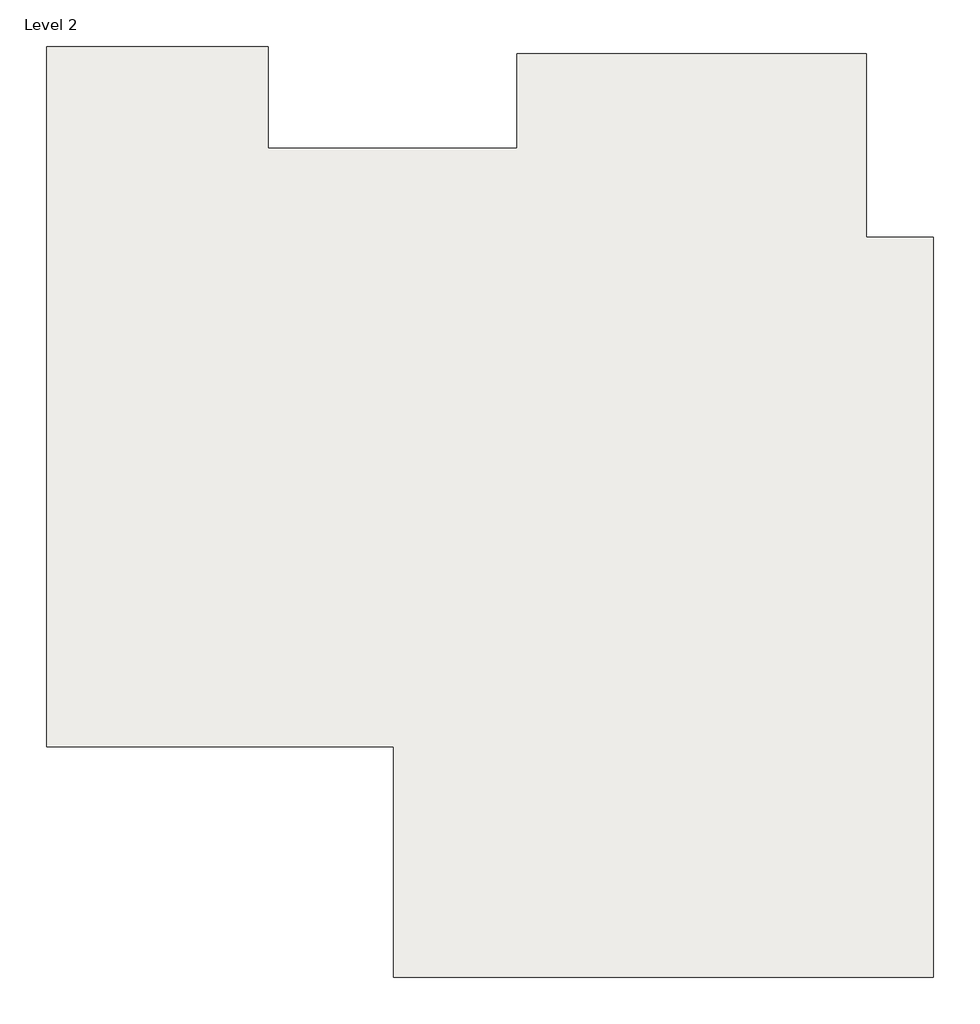
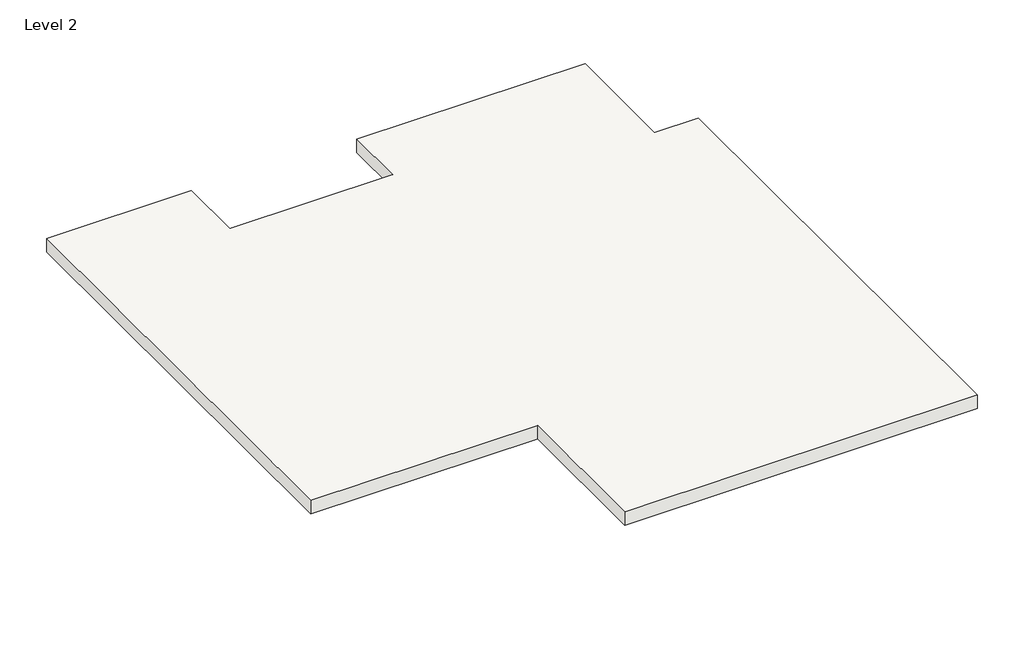
# One storey: 1 roof.
"""IFC4 building model written with IfcOpenShell, lengths in millimetres."""

from ifc_helpers import new_model, si_unit, frame, origin, place, context, project, spatial, polyline, outline, extrude, element, save

model = new_model("IFC4")

# Units and contexts
model_context = context("Model", 3, world=origin())
ifc_project = project(units=[si_unit("LENGTHUNIT", "METRE", prefix="MILLI")], contexts=[model_context])

# Site, building, storey
site = spatial("IfcSite", under=ifc_project)
building = spatial("IfcBuilding", under=site)
storey = spatial("IfcBuildingStorey", under=building, Name="Level 2", Elevation=3048.0)

# Roof
placement = place(None, origin())
element("IfcRoof", 1, ObjectType="Generic - 12\"", at=placement, inside=storey, context=model_context, shape_type="SweptSolid", body=[
    extrude(outline(polyline([(-12724.8234692, 10555.2116886), (-9626.0234692, 10555.2116886), (-9626.0234692, 9132.8116886), (-6146.2234692, 9132.8116886), (-6146.2234692, 10453.6116886), (-1269.4234692, 10453.6116886), (-1269.4234692, 7888.2116886), (-329.6234692, 7888.2116886), (-329.6234692, -2449.5883114), (-7873.4234692, -2449.5883114), (-7873.4234692, 776.2116886), (-12724.8234692, 776.2116886), (-12724.8234692, 10555.2116886)])), frame((0.0, 0.0, 3048.0), z_axis=(0.0, 0.0, 1.0), x_axis=(1.0, 0.0, 0.0)), (0.0, 0.0, 1.0), 304.8),
])

save(model, "model.ifc")

# Revit data of these elements
# Type "Generic - 12\""
#   Assembly Code = "B1020"
#   Layers, outside or top first: 1' - 0" "Brick, Soldier Course" (function 1)
# Element 1 (IfcRoof, "Generic - 12\"")
#   built-in parameter 1001705 = 11 (stored number, unit not read)
#   built-in parameter 1001710 = 33615
#   Phase Created = New Construction
#   Materials on its faces: "Brick, Soldier Course"
# Materials
#   "Brick, Soldier Course": class "Masonry", colour RGB 170 98 104, transparency 0, Description = "Common brick soldier coursed", Cost = 0
